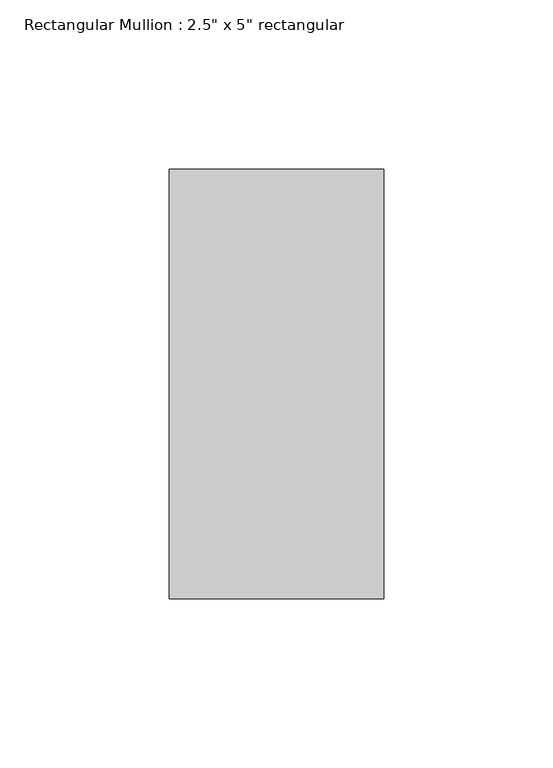
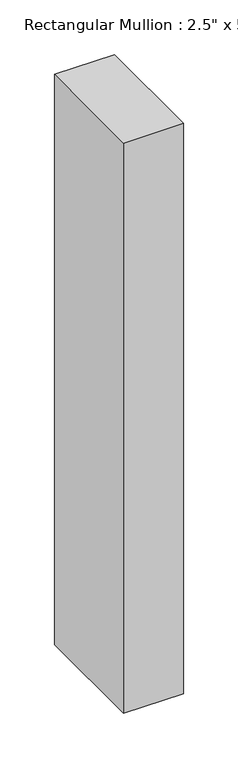
"""IFC4 building model written with IfcOpenShell, lengths in millimetres: member geometry."""

from ifc_helpers import new_model, si_unit, frame, origin, place, context, project, spatial, polyline, outline, extrude, source, transform, mapped, element, save


def member_04adda39(model_context):
    return source(origin(), model_context, "Body", "SweptSolid", [
        extrude(outline(polyline([(0.0, 63.5), (0.0, -63.5), (-63.5, -63.5), (-63.5, 63.5), (0.0, 63.5)])), frame((0.0, 0.0, -638.175), z_axis=(0.0, 0.0, 1.0), x_axis=(1.0, 0.0, 0.0)), (0.0, 0.0, 1.0), 638.175),
    ])


if __name__ == "__main__":
    model = new_model("IFC4")
    model_context = context("Model", 3, world=origin())
    ifc_project = project(units=[si_unit("LENGTHUNIT", "METRE", prefix="MILLI")], contexts=[model_context])
    site = spatial("IfcSite", under=ifc_project)
    building = spatial("IfcBuilding", under=site)
    placement = place(None, origin())
    member_shape = member_04adda39(model_context)
    element("IfcMember", 1, ObjectType="Rectangular Mullion : 2.5\" x 5\" rectangular", at=placement, inside=building, context=model_context, shape_type="MappedRepresentation", body=[
        mapped(member_shape, transform((0.0, 0.0, 0.0), x_axis=(1.0, 0.0, 0.0), y_axis=(0.0, 1.0, 0.0), z_axis=(0.0, 0.0, 1.0))),
    ])
    save(model, "model.ifc")

# Revit data of these elements
# Type "Rectangular Mullion : 2.5\" x 5\" rectangular"
#   built-in parameter 1007304 = 0.416667 (stored number, unit not read)
#   built-in parameter 1007301 = 0.104167 (stored number, unit not read)
#   built-in parameter 1007300 = 0.104167 (stored number, unit not read)
# Element 1 (IfcMember, "Rectangular Mullion : 2.5\" x 5\" rectangular")
#   Materials on its faces: "Aluminum"
# Materials
#   "Aluminum": class "Metal", colour RGB 247 247 247, transparency 0, Description = "Aluminum 6061", Cost = 0
